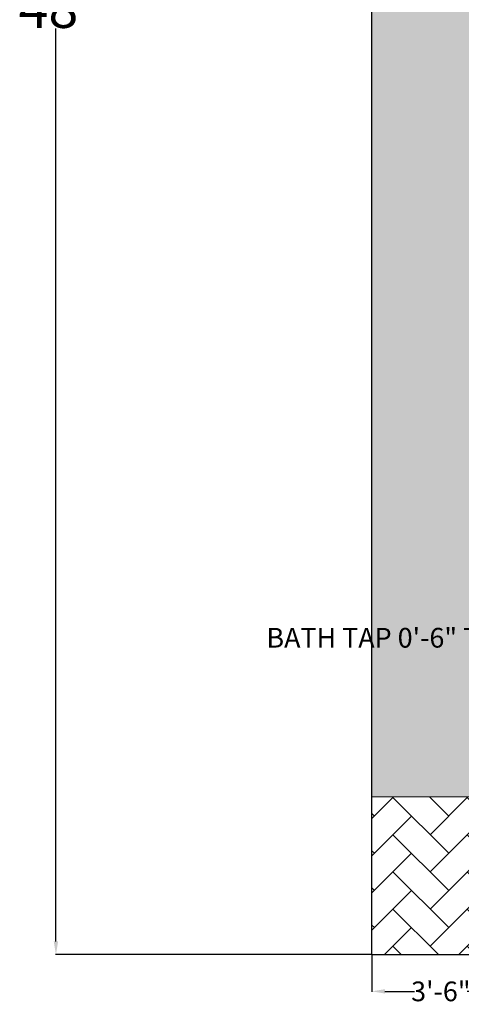
# Model space of a CAD drawing. Units: inches. Extents: x 803 to 1513, y 275 to 951.
# Tile 1 of 10: x 803 to 937, y 299 to 599. Entities that reach past the tile are written whole.
import ezdxf

# ---------------------------------------------------------------- set-up
doc = ezdxf.new("R2010")
doc.units = ezdxf.units.IN
doc.header["$MEASUREMENT"] = 0
for name, color, linetype, lineweight in [('C-PROP', 7, 'Continuous', 25), ('C-SITE', 8, 'Continuous', 18), ('C-SITE-PATT', 9, 'Continuous', 13), ('dim', 1, 'Continuous', 18)]:
    doc.layers.add(name, color=color, linetype=linetype, lineweight=lineweight)
doc.styles.get("Standard").update_dxf_attribs({"font": 'arial.ttf'})
doc.dimstyles.get("Standard").update_dxf_attribs({"dimtxt": 6, "dimasz": 4, "dimexe": 0.18, "dimexo": 0.0625, "dimgap": 0.09, "dimtad": 0, "dimtih": 1, "dimtoh": 1, "dimdec": 0, "dimzin": 0, "dimdsep": 46, "dimlunit": 3, "dimtxsty": 'Standard', "dimcen": 0.09, "dimadec": 0, "dimazin": 0, "dimtfac": 1, "dimtdec": 0, "dimtofl": 0, "dimtmove": 0, "dimatfit": 3, "dimfxl": 1, "dimtolj": 1, "dimtzin": 0, "dimarcsym": 0})

# ---------------------------------------------------------------- blocks, each defined once
blk = doc.blocks.new('*D50')
at = {"layer": 'Defpoints', "color": 0, "transparency": 16777216}
for p in [(910, 890.25), (813.84, 314.25), (910, 314.25)]:
    blk.add_point(p, dxfattribs=at)
at = {"layer": 'dim', "color": 0, "lineweight": -2, "transparency": 16777216}
for p, q in [((909.94, 890.25), (813.66, 890.25)), ((813.84, 886.25), (813.84, 608.47)), ((813.84, 318.25), (813.84, 596.03)), ((909.94, 314.25), (813.66, 314.25))]:
    blk.add_line(p, q, dxfattribs=at)
at = {"layer": 'dim', "color": 0, "transparency": 16777216}
for points in [[(813.17, 886.25), (814.51, 886.25), (813.84, 890.25)], [(813.17, 318.25), (814.51, 318.25), (813.84, 314.25)]]:
    blk.add_solid(points, dxfattribs=at)
at = {"layer": 'dim', "color": 0, "transparency": 16777216, "insert": (813.84, 602.25), "char_height": 6, "attachment_point": 5}
blk.add_mtext("\\A1;{\\H2x;48'}", dxfattribs=at)
blk = doc.blocks.new('*D56')
at = {"layer": 'Defpoints', "color": 0, "transparency": 16777216}
for p in [(910, 314.25), (952, 314.25), (910, 303.05)]:
    blk.add_point(p, dxfattribs=at)
at = {"layer": 'dim', "color": 0, "lineweight": -2, "transparency": 16777216}
for p, q in [((910, 314.19), (910, 302.87)), ((952, 314.19), (952, 302.87)), ((914, 303.05), (922.94, 303.05)), ((948, 303.05), (939.06, 303.05))]:
    blk.add_line(p, q, dxfattribs=at)
at = {"layer": 'dim', "color": 0, "transparency": 16777216}
for points in [[(914, 303.72), (914, 302.39), (910, 303.05)], [(948, 303.72), (948, 302.39), (952, 303.05)]]:
    blk.add_solid(points, dxfattribs=at)
at = {"layer": 'dim', "color": 0, "transparency": 16777216, "insert": (931, 303.05), "char_height": 6, "attachment_point": 5}
blk.add_mtext('\\A1;3\'-6"', dxfattribs=at)
blk = doc.blocks.new('*D79')
at = {"layer": 'Defpoints', "color": 0, "transparency": 16777216}
for p in [(961, 424.66), (960.1, 418.66), (961, 418.66)]:
    blk.add_point(p, dxfattribs=at)
at = {"layer": 'dim', "color": 0, "lineweight": -2, "transparency": 16777216}
for p, q in [((960.1, 428.66), (960.1, 432.66)), ((960.94, 424.66), (959.92, 424.66)), ((960.94, 418.66), (959.92, 418.66)), ((960.1, 414.66), (960.1, 410.66)), ((960.1, 410.66), (956.1, 410.66))]:
    blk.add_line(p, q, dxfattribs=at)
at = {"layer": 'dim', "color": 0, "transparency": 16777216}
for points in [[(959.43, 428.66), (960.77, 428.66), (960.1, 424.66)], [(959.43, 414.66), (960.77, 414.66), (960.1, 418.66)]]:
    blk.add_solid(points, dxfattribs=at)
at = {"layer": 'dim', "color": 0, "transparency": 16777216, "insert": (916.2, 410.66), "char_height": 6, "attachment_point": 5}
blk.add_mtext('\\A1;BATH TAP 0\'-6" TYP.', dxfattribs=at)

msp = doc.modelspace()

# ---------------------------------------------------------------- hatches: boundary and pattern name
at = {"layer": 'C-SITE-PATT'}
h = msp.add_hatch(dxfattribs=at)
h.set_pattern_fill('CROSS', color=256, scale=8)
h.paths.add_polyline_path([(952, 890.25), (910, 890.25), (910, 842.25), (952, 842.25)])
h.paths.add_polyline_path([(952, 842.25), (910, 842.25), (910, 362.25), (952, 362.25)])
h.paths.add_polyline_path([(1082.35, 890.25), (952, 890.25), (952, 842.25), (1082.35, 842.25)])
h.paths.add_polyline_path([(1432, 890.25), (1301.5, 890.25), (1301.5, 842.25), (1432, 842.25)])
h.paths.add_polyline_path([(1474, 890.25), (1432, 890.25), (1432, 842.25), (1474, 842.25)])
h.paths.add_polyline_path([(1474, 842.25), (1432, 842.25), (1432, 716.25), (1432, 362.25), (1474, 362.25)])
h.paths.add_polyline_path([(938.78, 396.85), (953.16, 396.85), (953.16, 421.58), (938.78, 421.58)], flags=9)
h.paths.add_polyline_path([(937.82, 612.92), (952.2, 612.92), (952.2, 637.65), (937.82, 637.65)], flags=9)
h.paths.add_polyline_path([(934.99, 667.62), (949.37, 667.62), (949.37, 692.35), (934.99, 692.35)], flags=24)
h.paths.add_polyline_path([(937.65, 500.72), (955.76, 500.72), (955.76, 525.45), (937.65, 525.45)], flags=9)
h.paths.add_polyline_path([(935.15, 758.83), (953.26, 758.83), (953.26, 783.56), (935.15, 783.56)], flags=9)
h.paths.add_polyline_path([(1011, 836.25), (1029.11, 836.25), (1029.11, 860.97), (1011, 860.97)], flags=9)
h.paths.add_polyline_path([(1346.52, 836.25), (1364.63, 836.25), (1364.63, 860.97), (1346.52, 860.97)], flags=9)
h.paths.add_polyline_path([(1430.4, 388.1), (1444.78, 388.1), (1444.78, 412.82), (1430.4, 412.82)], flags=9)
h.paths.add_polyline_path([(1429.9, 612.17), (1444.28, 612.17), (1444.28, 636.89), (1429.9, 636.89)], flags=9)
h.paths.add_polyline_path([(1429.47, 667.86), (1443.85, 667.86), (1443.85, 692.59), (1429.47, 692.59)], flags=9)
h.paths.add_polyline_path([(1431.88, 500.79), (1449.99, 500.79), (1449.99, 525.52), (1431.88, 525.52)], flags=9)
h.paths.add_polyline_path([(1429.97, 762.25), (1448.08, 762.25), (1448.08, 786.98), (1429.97, 786.98)], flags=9)
h = msp.add_hatch(dxfattribs=at)
h.set_pattern_fill('AR-HBONE', color=256, scale=2)
h.paths.add_polyline_path([(1432, 362.25), (952, 362.25), (952, 314.25), (1432, 314.25)])
h.paths.add_polyline_path([(952, 362.25), (910, 362.25), (910, 314.25), (952, 314.25)])
h.paths.add_polyline_path([(1474, 362.25), (1432, 362.25), (1432, 314.25), (1474, 314.25)])

# ---------------------------------------------------------------- linework, layer by layer
at = {"layer": 'C-PROP'}
for q in [(910, 890.25), (1474, 314.25)]:
    msp.add_line((910, 314.25), q, dxfattribs=at)
at = {"layer": 'C-SITE'}
msp.add_line((910, 362.25), (1474, 362.25), dxfattribs=at)

# ---------------------------------------------------------------- dimensions: what is measured, and where the dimension line sits
at = {"layer": 'dim'}
for base, p1, p2, angle, text, override, picture, middle in [((813.84, 314.25), (910, 890.25), (910, 314.25), 90, '{\\H2x;<>}', {"dimclrd": 0, "dimclre": 0, "dimclrt": 0}, '*D50', (813.84, 602.25)), ((960.1, 418.66), (961, 424.66), (961, 418.66), 270, 'BATH TAP <> TYP.', {"dimdec": 1, "dimlfac": 1, "dimrnd": 0, "dimzin": 1, "dimdsep": 46, "dimlunit": 4, "dimfrac": 2}, '*D79', (916.2, 410.66))]:
    dim = msp.add_linear_dim(base=base, p1=p1, p2=p2, angle=angle, text=text, dimstyle='Standard', override=override, dxfattribs=at)
    dim.commit()
    dim.dimension.update_dxf_attribs({"geometry": picture, "text_midpoint": middle})
dim = msp.add_linear_dim(base=(910, 303.05), p1=(952, 314.25), p2=(910, 314.25), dimstyle='Standard', override={"dimclrd": 0, "dimclre": 0, "dimclrt": 0}, dxfattribs=at)
dim.commit()
dim.dimension.update_dxf_attribs({"geometry": '*D56', "text_midpoint": (931, 303.05)})

doc.saveas('drawing.dxf')
